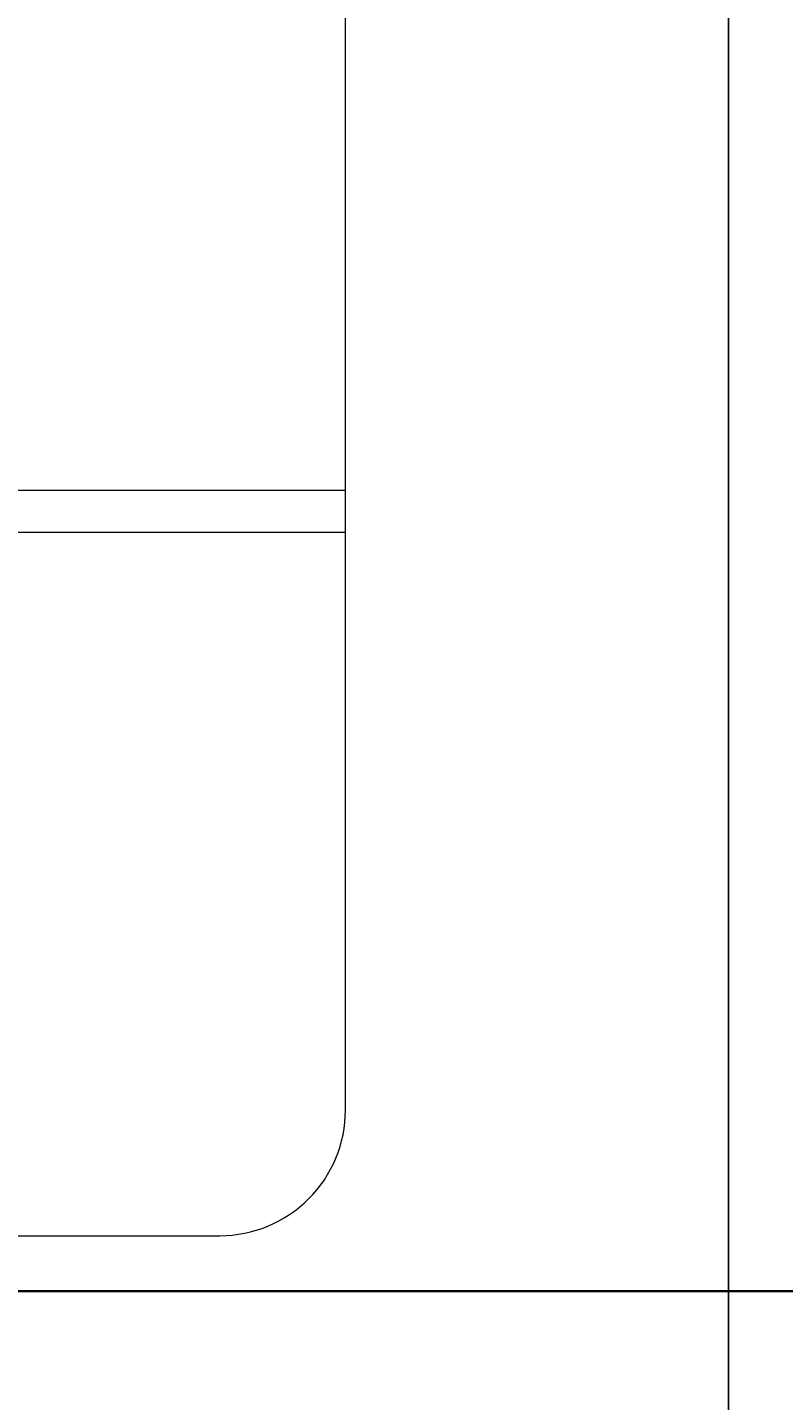
# Model space of a CAD drawing. Units: inches. Extents: x -61 to 1599, y -1316 to 257.
# Tile 119 of 204: x 161 to 181, y -10 to 27. Entities that reach past the tile are written whole.
import ezdxf

# ---------------------------------------------------------------- set-up
doc = ezdxf.new("R2010")
doc.units = ezdxf.units.IN
doc.header["$MEASUREMENT"] = 0
for name, color, linetype, lineweight in [('A-ANNO-DIMS', 2, 'Continuous', 18), ('FURNITURE', 83, 'Continuous', 18), ('WALLS', 4, 'Continuous', 35)]:
    doc.layers.add(name, color=color, linetype=linetype, lineweight=lineweight)
doc.styles.get("Standard").update_dxf_attribs({"font": 'arial.ttf'})
doc.dimstyles.get("Standard").update_dxf_attribs({"dimtxt": 0.18, "dimasz": 0.18, "dimexe": 0.18, "dimexo": 0.0625, "dimgap": 0.09, "dimtad": 0, "dimtih": 1, "dimtoh": 1, "dimdec": 0, "dimzin": 0, "dimdsep": 46, "dimlunit": 3, "dimtxsty": 'Standard', "dimcen": 0.09, "dimadec": 0, "dimazin": 0, "dimtfac": 1, "dimtdec": 0, "dimtofl": 0, "dimtmove": 0, "dimatfit": 3, "dimfxl": 1, "dimtolj": 1, "dimtzin": 0, "dimarcsym": 0})

# ---------------------------------------------------------------- blocks, each defined once
blk = doc.blocks.new('BED-DOUBLE')
for p, q in [((1.272, 20.467), (70.263, 20.467)), ((1.272, 19.317), (70.263, 19.317))]:
    blk.add_line(p, q)
blk.add_lwpolyline([(1.272, 88.537), (1.272, 3.449, 0.414214), (4.722, 0), (66.813, 0, 0.414214), (70.263, 3.449), (70.263, 88.537, 0.414214), (66.813, 91.987), (4.722, 91.987, 0.414214)], format="xyb", close=True)
blk = doc.blocks.new('*D687')
at = {"layer": 'A-ANNO-DIMS', "color": 0, "lineweight": -2, "transparency": 16777216}
for p, q in [((289.418, 181.677), (-61.077, 181.677)), ((-60.897, 181.497), (-60.897, -528.952)), ((-60.897, -1239.765), (-60.897, -529.316)), ((319.64, -1239.945), (-61.077, -1239.945))]:
    blk.add_line(p, q, dxfattribs=at)
at = {"layer": 'A-ANNO-DIMS', "color": 0, "transparency": 16777216}
for points in [[(-60.927, 181.497), (-60.867, 181.497), (-60.897, 181.677)], [(-60.927, -1239.765), (-60.867, -1239.765), (-60.897, -1239.945)]]:
    blk.add_solid(points, dxfattribs=at)
at = {"layer": 'DEFPOINTS', "color": 0, "transparency": 16777216}
for p in [(289.481, 181.677), (-60.897, -1239.945), (319.703, -1239.945)]:
    blk.add_point(p, dxfattribs=at)
at = {"layer": 'A-ANNO-DIMS', "color": 0, "transparency": 16777216, "insert": (-60.897, -529.134), "char_height": 0.18, "attachment_point": 5}
blk.add_mtext('\\A1;1421.6', dxfattribs=at)
blk = doc.blocks.new('*D700')
at = {"layer": 'A-ANNO-DIMS', "color": 0, "lineweight": -2, "transparency": 16777216}
for p, q in [((14.703, -616.882), (14.703, 257.457)), ((14.883, 257.277), (96.772, 257.277)), ((179.572, 257.277), (97.683, 257.277)), ((179.752, -616.882), (179.752, 257.457))]:
    blk.add_line(p, q, dxfattribs=at)
at = {"layer": 'A-ANNO-DIMS', "color": 0, "transparency": 16777216}
for points in [[(14.883, 257.307), (14.883, 257.247), (14.703, 257.277)], [(179.572, 257.307), (179.572, 257.247), (179.752, 257.277)]]:
    blk.add_solid(points, dxfattribs=at)
at = {"layer": 'DEFPOINTS', "color": 0, "transparency": 16777216}
for p in [(179.752, 257.277), (14.703, -616.945), (179.752, -616.945)]:
    blk.add_point(p, dxfattribs=at)
at = {"layer": 'A-ANNO-DIMS', "color": 0, "transparency": 16777216, "insert": (97.227, 257.277), "char_height": 0.18, "attachment_point": 5}
blk.add_mtext('\\A1;165.05', dxfattribs=at)

msp = doc.modelspace()

# ---------------------------------------------------------------- linework, layer by layer
at = {"layer": 'WALLS'}
msp.add_line((87.7028, -7.3229), (185.2611, -7.3229), dxfattribs=at)

# ---------------------------------------------------------------- block references
at = {"layer": 'FURNITURE'}
msp.add_blockref('BED-DOUBLE', (98.977, -5.797), dxfattribs=at)

# ---------------------------------------------------------------- dimensions: what is measured, and where the dimension line sits
at = {"layer": 'A-ANNO-DIMS'}
dim = msp.add_linear_dim(base=(179.7521, 257.2771), p1=(14.7028, -616.9446), p2=(179.7521, -616.9446), dimstyle='Standard', override={"dimdec": 2, "dimlfac": 1, "dimrnd": 0, "dimzin": 0, "dimdsep": 46, "dimlunit": 2}, dxfattribs=at)
dim.commit()
dim.dimension.update_dxf_attribs({"geometry": '*D700', "text_midpoint": (97.2274, 257.2771)})
dim = msp.add_linear_dim(base=(-60.8972, -1239.9446), p1=(289.4807, 181.6771), p2=(319.7028, -1239.9446), angle=90, dimstyle='Standard', override={"dimdec": 1, "dimlfac": 1, "dimrnd": 0, "dimzin": 0, "dimdsep": 46, "dimlunit": 2}, dxfattribs=at)
dim.commit()
dim.dimension.update_dxf_attribs({"geometry": '*D687', "text_midpoint": (-60.8972, -529.1337)})

doc.saveas('drawing.dxf')
